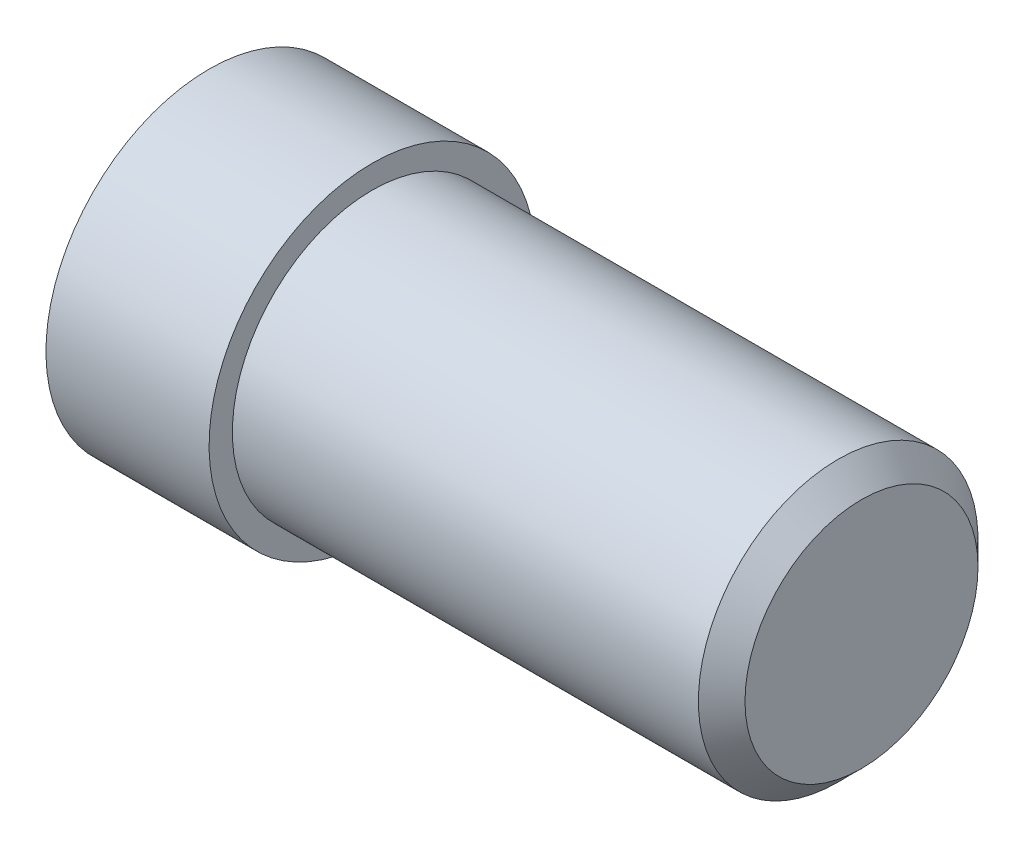
from build123d import *

# Parameters (mm, degrees)
SHANK_END_CHAMFER_1X45_SIZE = 1


with BuildPart() as part:
    # Bolt Profile Sketch → Bolt Body Revolve (revolve)
    with BuildSketch(Plane.XY):
        Polygon((0, 0), (0, 6), (-21, 6), (-21, 7), (-28, 7), (-28, 0), align=None)
    revolve(axis=Axis((0, 0, 0), (-1, 0, 0)))

    # Shank End Chamfer 1x45
    shank_end_chamfer_1x45_edges = [part.edges().sort_by_distance(p)[0] for p in [
        (0, -6, 0),
    ]]
    chamfer(shank_end_chamfer_1x45_edges, length=SHANK_END_CHAMFER_1X45_SIZE)


solid = part.part
